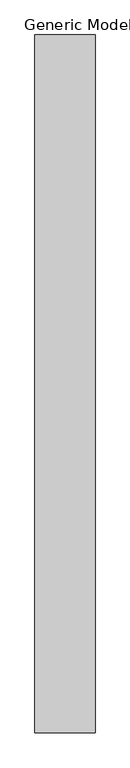
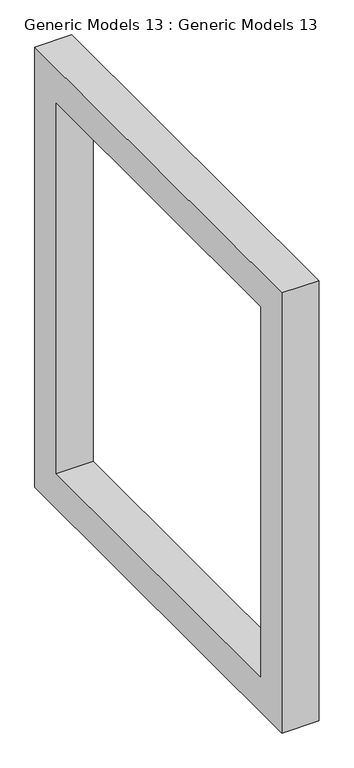
"""IFC4 building model written with IfcOpenShell, lengths in millimetres: proxy geometry, Generic Models 13 : Generic Models 13."""

from ifc_helpers import new_model, si_unit, frame, origin, place, context, project, spatial, polyline, outline, extrude, source, transform, mapped, element, save


def generic_models_13_generic_models_13_77cabad3(model_context):
    return source(origin(), model_context, "Body", "SweptSolid", [
        extrude(outline(polyline([(3084.8672538, 5740.4), (3084.8672538, 4140.2), (1611.6672538, 4140.2), (1611.6672538, 5740.4), (3084.8672538, 5740.4)]), holes=[polyline([(2957.8672538, 5613.4), (1738.6672538, 5613.4), (1738.6672538, 4267.2), (2957.8672538, 4267.2), (2957.8672538, 5613.4)])]), frame((-2408.3482439, 0.0, 0.0), z_axis=(1.0, 0.0, 0.0), x_axis=(0.0, 1.0, 0.0)), (0.0, 0.0, 1.0), 127.0),
    ])


if __name__ == "__main__":
    model = new_model("IFC4")
    model_context = context("Model", 3, world=origin())
    ifc_project = project(units=[si_unit("LENGTHUNIT", "METRE", prefix="MILLI")], contexts=[model_context])
    site = spatial("IfcSite", under=ifc_project)
    building = spatial("IfcBuilding", under=site)
    placement = place(None, origin())
    generic_models_13_generic_models_13_shape = generic_models_13_generic_models_13_77cabad3(model_context)
    element("IfcBuildingElementProxy", 1, Name="Generic Models 13 : Generic Models 13", ObjectType="Generic Models 13 : Generic Models 13", at=placement, inside=building, context=model_context, shape_type="MappedRepresentation", body=[
        mapped(generic_models_13_generic_models_13_shape, transform((0.0, 0.0, 0.0), x_axis=(1.0, 0.0, 0.0), y_axis=(0.0, 1.0, 0.0), z_axis=(0.0, 0.0, 1.0))),
    ])
    save(model, "model.ifc")

# Revit data of these elements
# Element 1 (IfcBuildingElementProxy, "Generic Models 13 : Generic Models 13")
#   Materials on its faces: "BLACK"
# Materials
#   "BLACK": class "Generic", colour RGB 120 120 120, transparency 0, Cost = 0
